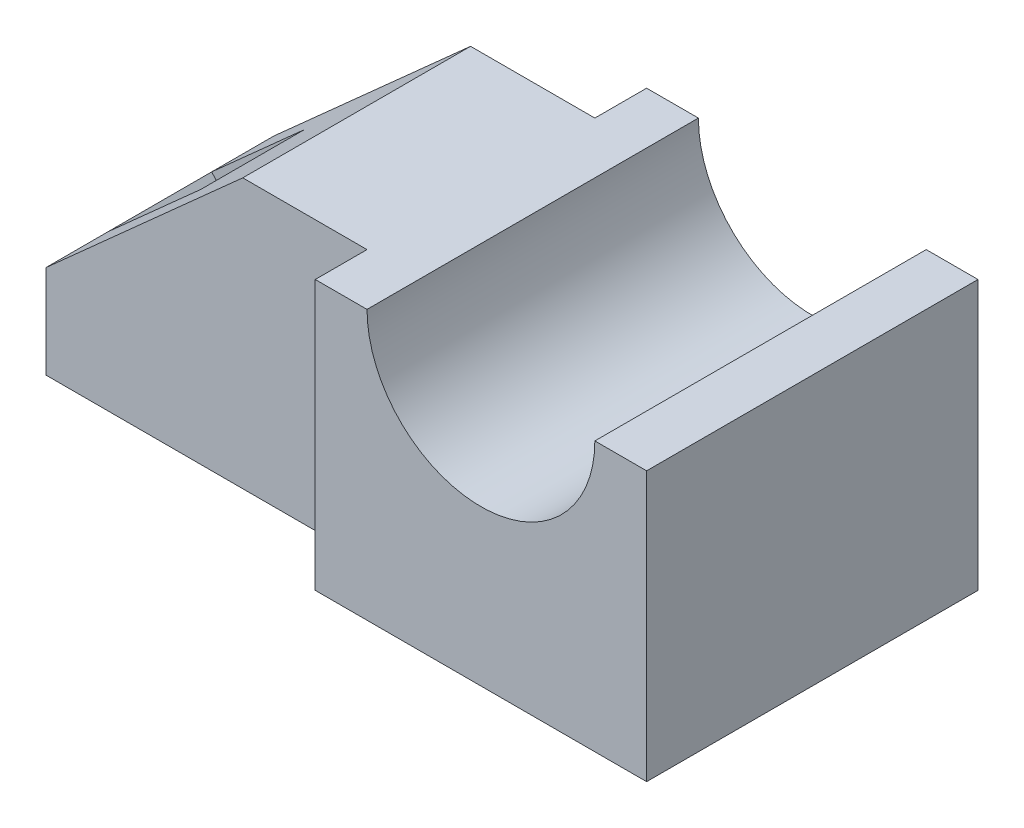
ISO-10303-21;
HEADER;
FILE_DESCRIPTION(('STEP AP214'),'2;1');
FILE_NAME('part.step','',(''),(''),'','','');
FILE_SCHEMA(('AUTOMOTIVE_DESIGN { 1 0 10303 214 1 1 1 1 }'));
ENDSEC;
DATA;
#1=APPLICATION_CONTEXT('core data for automotive mechanical design processes');
#2=APPLICATION_PROTOCOL_DEFINITION('international standard','automotive_design',2000,#1);
#3=PRODUCT_CONTEXT('',#1,'mechanical');
#4=PRODUCT('Part','Part','',(#3));
#5=PRODUCT_RELATED_PRODUCT_CATEGORY('part','',(#4));
#6=PRODUCT_DEFINITION_FORMATION('','',#4);
#7=PRODUCT_DEFINITION_CONTEXT('part definition',#1,'design');
#8=PRODUCT_DEFINITION('design','',#6,#7);
#9=PRODUCT_DEFINITION_SHAPE('','',#8);
#10=(LENGTH_UNIT() NAMED_UNIT(*) SI_UNIT(.MILLI.,.METRE.));
#11=(NAMED_UNIT(*) PLANE_ANGLE_UNIT() SI_UNIT($,.RADIAN.));
#12=(NAMED_UNIT(*) SI_UNIT($,.STERADIAN.) SOLID_ANGLE_UNIT());
#13=UNCERTAINTY_MEASURE_WITH_UNIT(LENGTH_MEASURE(1.E-05),#10,'distance_accuracy_value','');
#14=(GEOMETRIC_REPRESENTATION_CONTEXT(3) GLOBAL_UNCERTAINTY_ASSIGNED_CONTEXT((#13)) GLOBAL_UNIT_ASSIGNED_CONTEXT((#10,
#11,#12)) REPRESENTATION_CONTEXT('',''));
#15=CARTESIAN_POINT('',(0.,0.,0.));
#16=DIRECTION('',(0.,0.,1.));
#17=DIRECTION('',(1.,0.,0.));
#18=AXIS2_PLACEMENT_3D('',#15,#16,#17);
#19=CARTESIAN_POINT('',(-16.,13.,16.));
#20=DIRECTION('',(1.,0.,0.));
#21=DIRECTION('',(0.,1.,0.));
#22=AXIS2_PLACEMENT_3D('',#19,#20,#21);
#23=PLANE('',#22);
#24=DIRECTION('',(0.,1.,0.));
#25=VECTOR('',#24,1.);
#26=CARTESIAN_POINT('',(-16.,13.,11.));
#27=LINE('',#26,#25);
#28=CARTESIAN_POINT('',(-16.,-13.,11.));
#29=VERTEX_POINT('',#28);
#30=CARTESIAN_POINT('',(-16.,13.,11.));
#31=VERTEX_POINT('',#30);
#32=EDGE_CURVE('E285',#29,#31,#27,.T.);
#33=ORIENTED_EDGE('',*,*,#32,.F.);
#34=DIRECTION('',(0.,0.,-1.));
#35=VECTOR('',#34,1.);
#36=CARTESIAN_POINT('',(-16.,-13.,16.));
#37=LINE('',#36,#35);
#38=CARTESIAN_POINT('',(-16.,-13.,16.));
#39=VERTEX_POINT('',#38);
#40=EDGE_CURVE('E220',#39,#29,#37,.T.);
#41=ORIENTED_EDGE('',*,*,#40,.F.);
#42=DIRECTION('',(0.,-1.,0.));
#43=VECTOR('',#42,1.);
#44=CARTESIAN_POINT('',(-16.,13.,16.));
#45=LINE('',#44,#43);
#46=CARTESIAN_POINT('',(-16.,13.,16.));
#47=VERTEX_POINT('',#46);
#48=EDGE_CURVE('E198',#47,#39,#45,.T.);
#49=ORIENTED_EDGE('',*,*,#48,.F.);
#50=DIRECTION('',(0.,0.,-1.));
#51=VECTOR('',#50,1.);
#52=CARTESIAN_POINT('',(-16.,13.,16.));
#53=LINE('',#52,#51);
#54=EDGE_CURVE('E222',#47,#31,#53,.T.);
#55=ORIENTED_EDGE('',*,*,#54,.T.);
#56=EDGE_LOOP('',(#33,#41,#49,#55));
#57=FACE_BOUND('',#56,.T.);
#58=ADVANCED_FACE('F39',(#57),#23,.F.);
#59=CARTESIAN_POINT('',(16.,13.,16.));
#60=DIRECTION('',(-1.,0.,0.));
#61=DIRECTION('',(0.,-1.,0.));
#62=AXIS2_PLACEMENT_3D('',#59,#60,#61);
#63=PLANE('',#62);
#64=DIRECTION('',(0.,1.,0.));
#65=VECTOR('',#64,1.);
#66=CARTESIAN_POINT('',(16.,13.,-16.));
#67=LINE('',#66,#65);
#68=CARTESIAN_POINT('',(16.,-13.,-16.));
#69=VERTEX_POINT('',#68);
#70=CARTESIAN_POINT('',(16.,13.,-16.));
#71=VERTEX_POINT('',#70);
#72=EDGE_CURVE('E179',#69,#71,#67,.T.);
#73=ORIENTED_EDGE('',*,*,#72,.T.);
#74=DIRECTION('',(0.,0.,-1.));
#75=VECTOR('',#74,1.);
#76=CARTESIAN_POINT('',(16.,13.,16.));
#77=LINE('',#76,#75);
#78=CARTESIAN_POINT('',(16.,13.,16.));
#79=VERTEX_POINT('',#78);
#80=EDGE_CURVE('E11',#79,#71,#77,.T.);
#81=ORIENTED_EDGE('',*,*,#80,.F.);
#82=DIRECTION('',(0.,1.,0.));
#83=VECTOR('',#82,1.);
#84=CARTESIAN_POINT('',(16.,13.,16.));
#85=LINE('',#84,#83);
#86=CARTESIAN_POINT('',(16.,-13.,16.));
#87=VERTEX_POINT('',#86);
#88=EDGE_CURVE('E186',#87,#79,#85,.T.);
#89=ORIENTED_EDGE('',*,*,#88,.F.);
#90=DIRECTION('',(0.,0.,-1.));
#91=VECTOR('',#90,1.);
#92=CARTESIAN_POINT('',(16.,-13.,16.));
#93=LINE('',#92,#91);
#94=EDGE_CURVE('E199',#87,#69,#93,.T.);
#95=ORIENTED_EDGE('',*,*,#94,.T.);
#96=EDGE_LOOP('',(#73,#81,#89,#95));
#97=FACE_BOUND('',#96,.T.);
#98=ADVANCED_FACE('F41',(#97),#63,.F.);
#99=CARTESIAN_POINT('',(11.,13.,16.));
#100=DIRECTION('',(0.,-1.,0.));
#101=DIRECTION('',(1.,0.,0.));
#102=AXIS2_PLACEMENT_3D('',#99,#100,#101);
#103=PLANE('',#102);
#104=DIRECTION('',(-1.,0.,0.));
#105=VECTOR('',#104,1.);
#106=CARTESIAN_POINT('',(11.,13.,-16.));
#107=LINE('',#106,#105);
#108=CARTESIAN_POINT('',(11.,13.,-16.));
#109=VERTEX_POINT('',#108);
#110=EDGE_CURVE('E201',#71,#109,#107,.T.);
#111=ORIENTED_EDGE('',*,*,#110,.T.);
#112=DIRECTION('',(0.,0.,-1.));
#113=VECTOR('',#112,1.);
#114=CARTESIAN_POINT('',(11.,13.,16.));
#115=LINE('',#114,#113);
#116=CARTESIAN_POINT('',(11.,13.,16.));
#117=VERTEX_POINT('',#116);
#118=EDGE_CURVE('E50',#117,#109,#115,.T.);
#119=ORIENTED_EDGE('',*,*,#118,.F.);
#120=DIRECTION('',(-1.,0.,0.));
#121=VECTOR('',#120,1.);
#122=CARTESIAN_POINT('',(11.,13.,16.));
#123=LINE('',#122,#121);
#124=EDGE_CURVE('E188',#79,#117,#123,.T.);
#125=ORIENTED_EDGE('',*,*,#124,.F.);
#126=ORIENTED_EDGE('',*,*,#80,.T.);
#127=EDGE_LOOP('',(#111,#119,#125,#126));
#128=FACE_BOUND('',#127,.T.);
#129=ADVANCED_FACE('F252',(#128),#103,.F.);
#130=CARTESIAN_POINT('',(0.,13.,16.));
#131=DIRECTION('',(0.,0.,-1.));
#132=DIRECTION('',(-1.,0.,0.));
#133=AXIS2_PLACEMENT_3D('',#130,#131,#132);
#134=CYLINDRICAL_SURFACE('',#133,11.);
#135=CARTESIAN_POINT('',(0.,13.,-16.));
#136=DIRECTION('',(0.,0.,-1.));
#137=DIRECTION('',(1.,0.,0.));
#138=AXIS2_PLACEMENT_3D('',#135,#136,#137);
#139=CIRCLE('',#138,11.);
#140=CARTESIAN_POINT('',(-11.,13.,-16.));
#141=VERTEX_POINT('',#140);
#142=EDGE_CURVE('E202',#109,#141,#139,.T.);
#143=ORIENTED_EDGE('',*,*,#142,.T.);
#144=DIRECTION('',(0.,0.,-1.));
#145=VECTOR('',#144,1.);
#146=CARTESIAN_POINT('',(-11.,13.,16.));
#147=LINE('',#146,#145);
#148=CARTESIAN_POINT('',(-11.,13.,16.));
#149=VERTEX_POINT('',#148);
#150=EDGE_CURVE('E224',#149,#141,#147,.T.);
#151=ORIENTED_EDGE('',*,*,#150,.F.);
#152=CARTESIAN_POINT('',(0.,13.,16.));
#153=DIRECTION('',(0.,0.,-1.));
#154=DIRECTION('',(1.,0.,0.));
#155=AXIS2_PLACEMENT_3D('',#152,#153,#154);
#156=CIRCLE('',#155,11.);
#157=EDGE_CURVE('E195',#117,#149,#156,.T.);
#158=ORIENTED_EDGE('',*,*,#157,.F.);
#159=ORIENTED_EDGE('',*,*,#118,.T.);
#160=EDGE_LOOP('',(#143,#151,#158,#159));
#161=FACE_BOUND('',#160,.T.);
#162=ADVANCED_FACE('F229',(#161),#134,.F.);
#163=CARTESIAN_POINT('',(-16.,13.,16.));
#164=DIRECTION('',(0.,-1.,0.));
#165=DIRECTION('',(1.,0.,0.));
#166=AXIS2_PLACEMENT_3D('',#163,#164,#165);
#167=PLANE('',#166);
#168=DIRECTION('',(-1.,0.,0.));
#169=VECTOR('',#168,1.);
#170=CARTESIAN_POINT('',(-16.,13.,-16.));
#171=LINE('',#170,#169);
#172=CARTESIAN_POINT('',(-16.,13.,-16.));
#173=VERTEX_POINT('',#172);
#174=EDGE_CURVE('E210',#141,#173,#171,.T.);
#175=ORIENTED_EDGE('',*,*,#174,.T.);
#176=CARTESIAN_POINT('',(-16.,13.,-11.));
#177=VERTEX_POINT('',#176);
#178=EDGE_CURVE('E219',#177,#173,#53,.T.);
#179=ORIENTED_EDGE('',*,*,#178,.F.);
#180=DIRECTION('',(-1.,0.,0.));
#181=VECTOR('',#180,1.);
#182=CARTESIAN_POINT('',(-16.,13.,-11.));
#183=LINE('',#182,#181);
#184=CARTESIAN_POINT('',(-28.,13.,-11.));
#185=VERTEX_POINT('',#184);
#186=EDGE_CURVE('E270',#177,#185,#183,.T.);
#187=ORIENTED_EDGE('',*,*,#186,.T.);
#188=DIRECTION('',(0.,0.,-1.));
#189=VECTOR('',#188,1.);
#190=CARTESIAN_POINT('',(-28.,13.,11.));
#191=LINE('',#190,#189);
#192=CARTESIAN_POINT('',(-28.,13.,11.));
#193=VERTEX_POINT('',#192);
#194=EDGE_CURVE('E178',#193,#185,#191,.T.);
#195=ORIENTED_EDGE('',*,*,#194,.F.);
#196=DIRECTION('',(-1.,0.,0.));
#197=VECTOR('',#196,1.);
#198=CARTESIAN_POINT('',(-16.,13.,11.));
#199=LINE('',#198,#197);
#200=EDGE_CURVE('E283',#31,#193,#199,.T.);
#201=ORIENTED_EDGE('',*,*,#200,.F.);
#202=ORIENTED_EDGE('',*,*,#54,.F.);
#203=DIRECTION('',(-1.,0.,0.));
#204=VECTOR('',#203,1.);
#205=CARTESIAN_POINT('',(-16.,13.,16.));
#206=LINE('',#205,#204);
#207=EDGE_CURVE('E192',#149,#47,#206,.T.);
#208=ORIENTED_EDGE('',*,*,#207,.F.);
#209=ORIENTED_EDGE('',*,*,#150,.T.);
#210=EDGE_LOOP('',(#175,#179,#187,#195,#201,#202,#208,#209));
#211=FACE_BOUND('',#210,.T.);
#212=ADVANCED_FACE('F241',(#211),#167,.F.);
#213=CARTESIAN_POINT('',(-16.,-13.,-11.));
#214=VERTEX_POINT('',#213);
#215=CARTESIAN_POINT('',(-16.,-13.,-16.));
#216=VERTEX_POINT('',#215);
#217=EDGE_CURVE('E216',#214,#216,#37,.T.);
#218=ORIENTED_EDGE('',*,*,#217,.F.);
#219=DIRECTION('',(0.,1.,0.));
#220=VECTOR('',#219,1.);
#221=CARTESIAN_POINT('',(-16.,13.,-11.));
#222=LINE('',#221,#220);
#223=EDGE_CURVE('E264',#214,#177,#222,.T.);
#224=ORIENTED_EDGE('',*,*,#223,.T.);
#225=ORIENTED_EDGE('',*,*,#178,.T.);
#226=DIRECTION('',(0.,-1.,0.));
#227=VECTOR('',#226,1.);
#228=CARTESIAN_POINT('',(-16.,13.,-16.));
#229=LINE('',#228,#227);
#230=EDGE_CURVE('E209',#173,#216,#229,.T.);
#231=ORIENTED_EDGE('',*,*,#230,.T.);
#232=EDGE_LOOP('',(#218,#224,#225,#231));
#233=FACE_BOUND('',#232,.T.);
#234=ADVANCED_FACE('F262',(#233),#23,.F.);
#235=CARTESIAN_POINT('',(-16.,-13.,16.));
#236=DIRECTION('',(0.,1.,0.));
#237=DIRECTION('',(0.,0.,1.));
#238=AXIS2_PLACEMENT_3D('',#235,#236,#237);
#239=PLANE('',#238);
#240=DIRECTION('',(-1.,0.,0.));
#241=VECTOR('',#240,1.);
#242=CARTESIAN_POINT('',(-16.,-13.,-5.));
#243=LINE('',#242,#241);
#244=CARTESIAN_POINT('',(-22.8452015360228,-13.,-5.));
#245=VERTEX_POINT('',#244);
#246=CARTESIAN_POINT('',(-38.9473684210526,-13.,-5.));
#247=VERTEX_POINT('',#246);
#248=EDGE_CURVE('E435',#245,#247,#243,.T.);
#249=ORIENTED_EDGE('',*,*,#248,.T.);
#250=DIRECTION('',(0.,0.,1.));
#251=VECTOR('',#250,1.);
#252=CARTESIAN_POINT('',(-38.9473684210526,-13.,16.));
#253=LINE('',#252,#251);
#254=CARTESIAN_POINT('',(-38.9473684210526,-13.,5.));
#255=VERTEX_POINT('',#254);
#256=EDGE_CURVE('E272',#247,#255,#253,.T.);
#257=ORIENTED_EDGE('',*,*,#256,.T.);
#258=DIRECTION('',(1.,0.,0.));
#259=VECTOR('',#258,1.);
#260=CARTESIAN_POINT('',(-16.,-13.,5.));
#261=LINE('',#260,#259);
#262=CARTESIAN_POINT('',(-22.8452015360228,-13.,5.));
#263=VERTEX_POINT('',#262);
#264=EDGE_CURVE('E155',#255,#263,#261,.T.);
#265=ORIENTED_EDGE('',*,*,#264,.T.);
#266=DIRECTION('',(0.,0.,-1.));
#267=VECTOR('',#266,1.);
#268=CARTESIAN_POINT('',(-22.8452015360228,-13.,16.));
#269=LINE('',#268,#267);
#270=EDGE_CURVE('E268',#263,#245,#269,.T.);
#271=ORIENTED_EDGE('',*,*,#270,.T.);
#272=EDGE_LOOP('',(#249,#257,#265,#271));
#273=FACE_BOUND('',#272,.T.);
#274=DIRECTION('',(1.,0.,0.));
#275=VECTOR('',#274,1.);
#276=CARTESIAN_POINT('',(-16.,-13.,-16.));
#277=LINE('',#276,#275);
#278=EDGE_CURVE('E189',#216,#69,#277,.T.);
#279=ORIENTED_EDGE('',*,*,#278,.T.);
#280=ORIENTED_EDGE('',*,*,#94,.F.);
#281=DIRECTION('',(1.,0.,0.));
#282=VECTOR('',#281,1.);
#283=CARTESIAN_POINT('',(-16.,-13.,16.));
#284=LINE('',#283,#282);
#285=EDGE_CURVE('E196',#39,#87,#284,.T.);
#286=ORIENTED_EDGE('',*,*,#285,.F.);
#287=ORIENTED_EDGE('',*,*,#40,.T.);
#288=DIRECTION('',(1.,0.,0.));
#289=VECTOR('',#288,1.);
#290=CARTESIAN_POINT('',(-47.,-13.,11.));
#291=LINE('',#290,#289);
#292=CARTESIAN_POINT('',(-47.,-13.,11.));
#293=VERTEX_POINT('',#292);
#294=EDGE_CURVE('E277',#293,#29,#291,.T.);
#295=ORIENTED_EDGE('',*,*,#294,.F.);
#296=DIRECTION('',(0.,0.,-1.));
#297=VECTOR('',#296,1.);
#298=CARTESIAN_POINT('',(-47.,-13.,11.));
#299=LINE('',#298,#297);
#300=CARTESIAN_POINT('',(-47.,-13.,-11.));
#301=VERTEX_POINT('',#300);
#302=EDGE_CURVE('E185',#293,#301,#299,.T.);
#303=ORIENTED_EDGE('',*,*,#302,.T.);
#304=DIRECTION('',(1.,0.,0.));
#305=VECTOR('',#304,1.);
#306=CARTESIAN_POINT('',(-47.,-13.,-11.));
#307=LINE('',#306,#305);
#308=EDGE_CURVE('E261',#301,#214,#307,.T.);
#309=ORIENTED_EDGE('',*,*,#308,.T.);
#310=ORIENTED_EDGE('',*,*,#217,.T.);
#311=EDGE_LOOP('',(#279,#280,#286,#287,#295,#303,#309,#310));
#312=FACE_BOUND('',#311,.T.);
#313=ADVANCED_FACE('F258',(#273,#312),#239,.F.);
#314=CARTESIAN_POINT('',(0.,13.,16.));
#315=DIRECTION('',(0.,0.,1.));
#316=DIRECTION('',(1.,0.,0.));
#317=AXIS2_PLACEMENT_3D('',#314,#315,#316);
#318=PLANE('',#317);
#319=ORIENTED_EDGE('',*,*,#88,.T.);
#320=ORIENTED_EDGE('',*,*,#124,.T.);
#321=ORIENTED_EDGE('',*,*,#157,.T.);
#322=ORIENTED_EDGE('',*,*,#207,.T.);
#323=ORIENTED_EDGE('',*,*,#48,.T.);
#324=ORIENTED_EDGE('',*,*,#285,.T.);
#325=EDGE_LOOP('',(#319,#320,#321,#322,#323,#324));
#326=FACE_BOUND('',#325,.T.);
#327=ADVANCED_FACE('F246',(#326),#318,.T.);
#328=CARTESIAN_POINT('',(0.,13.,-16.));
#329=DIRECTION('',(0.,0.,1.));
#330=DIRECTION('',(1.,0.,0.));
#331=AXIS2_PLACEMENT_3D('',#328,#329,#330);
#332=PLANE('',#331);
#333=ORIENTED_EDGE('',*,*,#72,.F.);
#334=ORIENTED_EDGE('',*,*,#278,.F.);
#335=ORIENTED_EDGE('',*,*,#230,.F.);
#336=ORIENTED_EDGE('',*,*,#174,.F.);
#337=ORIENTED_EDGE('',*,*,#142,.F.);
#338=ORIENTED_EDGE('',*,*,#110,.F.);
#339=EDGE_LOOP('',(#333,#334,#335,#336,#337,#338));
#340=FACE_BOUND('',#339,.T.);
#341=ADVANCED_FACE('F237',(#340),#332,.F.);
#342=CARTESIAN_POINT('',(-28.,13.,11.));
#343=DIRECTION('',(0.666794859469826,-0.745241313525099,0.));
#344=DIRECTION('',(0.745241313525099,0.666794859469826,0.));
#345=AXIS2_PLACEMENT_3D('',#342,#343,#344);
#346=PLANE('',#345);
#347=DIRECTION('',(0.,0.,-1.));
#348=VECTOR('',#347,1.);
#349=CARTESIAN_POINT('',(-47.,-4.,11.));
#350=LINE('',#349,#348);
#351=CARTESIAN_POINT('',(-47.,-4.,-5.));
#352=VERTEX_POINT('',#351);
#353=CARTESIAN_POINT('',(-47.,-4.,-11.));
#354=VERTEX_POINT('',#353);
#355=EDGE_CURVE('E180',#352,#354,#350,.T.);
#356=ORIENTED_EDGE('',*,*,#355,.F.);
#357=DIRECTION('',(-0.745241313525099,-0.666794859469826,0.));
#358=VECTOR('',#357,1.);
#359=CARTESIAN_POINT('',(-47.,-4.00000000000001,-5.));
#360=LINE('',#359,#358);
#361=CARTESIAN_POINT('',(-38.0571042376988,4.00153831363791,-5.));
#362=VERTEX_POINT('',#361);
#363=EDGE_CURVE('E65',#362,#352,#360,.T.);
#364=ORIENTED_EDGE('',*,*,#363,.F.);
#365=DIRECTION('',(0.,0.,-1.));
#366=VECTOR('',#365,1.);
#367=CARTESIAN_POINT('',(-38.0571042376988,4.00153831363791,-5.));
#368=LINE('',#367,#366);
#369=CARTESIAN_POINT('',(-38.0571042376988,4.00153831363791,5.));
#370=VERTEX_POINT('',#369);
#371=EDGE_CURVE('E171',#370,#362,#368,.T.);
#372=ORIENTED_EDGE('',*,*,#371,.F.);
#373=DIRECTION('',(0.745241313525099,0.666794859469826,0.));
#374=VECTOR('',#373,1.);
#375=CARTESIAN_POINT('',(-38.0571042376988,4.00153831363791,5.));
#376=LINE('',#375,#374);
#377=CARTESIAN_POINT('',(-47.,-4.00000000000001,5.));
#378=VERTEX_POINT('',#377);
#379=EDGE_CURVE('E149',#378,#370,#376,.T.);
#380=ORIENTED_EDGE('',*,*,#379,.F.);
#381=CARTESIAN_POINT('',(-47.,-4.,11.));
#382=VERTEX_POINT('',#381);
#383=EDGE_CURVE('E169',#382,#378,#350,.T.);
#384=ORIENTED_EDGE('',*,*,#383,.F.);
#385=DIRECTION('',(-0.745241313525099,-0.666794859469826,0.));
#386=VECTOR('',#385,1.);
#387=CARTESIAN_POINT('',(-28.,13.,11.));
#388=LINE('',#387,#386);
#389=EDGE_CURVE('E286',#193,#382,#388,.T.);
#390=ORIENTED_EDGE('',*,*,#389,.F.);
#391=ORIENTED_EDGE('',*,*,#194,.T.);
#392=DIRECTION('',(-0.745241313525099,-0.666794859469826,0.));
#393=VECTOR('',#392,1.);
#394=CARTESIAN_POINT('',(-28.,13.,-11.));
#395=LINE('',#394,#393);
#396=EDGE_CURVE('E269',#185,#354,#395,.T.);
#397=ORIENTED_EDGE('',*,*,#396,.T.);
#398=EDGE_LOOP('',(#356,#364,#372,#380,#384,#390,#391,#397));
#399=FACE_BOUND('',#398,.T.);
#400=ADVANCED_FACE('F167',(#399),#346,.F.);
#401=CARTESIAN_POINT('',(-47.,-4.,11.));
#402=DIRECTION('',(1.,0.,0.));
#403=DIRECTION('',(0.,0.,-1.));
#404=AXIS2_PLACEMENT_3D('',#401,#402,#403);
#405=PLANE('',#404);
#406=DIRECTION('',(0.,-1.,0.));
#407=VECTOR('',#406,1.);
#408=CARTESIAN_POINT('',(-47.,-4.,-11.));
#409=LINE('',#408,#407);
#410=EDGE_CURVE('E281',#354,#301,#409,.T.);
#411=ORIENTED_EDGE('',*,*,#410,.T.);
#412=ORIENTED_EDGE('',*,*,#302,.F.);
#413=DIRECTION('',(0.,-1.,0.));
#414=VECTOR('',#413,1.);
#415=CARTESIAN_POINT('',(-47.,-4.,11.));
#416=LINE('',#415,#414);
#417=EDGE_CURVE('E174',#382,#293,#416,.T.);
#418=ORIENTED_EDGE('',*,*,#417,.F.);
#419=ORIENTED_EDGE('',*,*,#383,.T.);
#420=DIRECTION('',(0.,0.,1.));
#421=VECTOR('',#420,1.);
#422=CARTESIAN_POINT('',(-47.,-4.00000000000001,-5.));
#423=LINE('',#422,#421);
#424=EDGE_CURVE('E160',#352,#378,#423,.T.);
#425=ORIENTED_EDGE('',*,*,#424,.F.);
#426=ORIENTED_EDGE('',*,*,#355,.T.);
#427=EDGE_LOOP('',(#411,#412,#418,#419,#425,#426));
#428=FACE_BOUND('',#427,.T.);
#429=ADVANCED_FACE('F172',(#428),#405,.F.);
#430=CARTESIAN_POINT('',(0.,0.,11.));
#431=DIRECTION('',(0.,0.,1.));
#432=DIRECTION('',(1.,0.,0.));
#433=AXIS2_PLACEMENT_3D('',#430,#431,#432);
#434=PLANE('',#433);
#435=ORIENTED_EDGE('',*,*,#32,.T.);
#436=ORIENTED_EDGE('',*,*,#200,.T.);
#437=ORIENTED_EDGE('',*,*,#389,.T.);
#438=ORIENTED_EDGE('',*,*,#417,.T.);
#439=ORIENTED_EDGE('',*,*,#294,.T.);
#440=EDGE_LOOP('',(#435,#436,#437,#438,#439));
#441=FACE_BOUND('',#440,.T.);
#442=ADVANCED_FACE('F300',(#441),#434,.T.);
#443=CARTESIAN_POINT('',(0.,0.,-11.));
#444=DIRECTION('',(0.,0.,1.));
#445=DIRECTION('',(1.,0.,0.));
#446=AXIS2_PLACEMENT_3D('',#443,#444,#445);
#447=PLANE('',#446);
#448=ORIENTED_EDGE('',*,*,#223,.F.);
#449=ORIENTED_EDGE('',*,*,#308,.F.);
#450=ORIENTED_EDGE('',*,*,#410,.F.);
#451=ORIENTED_EDGE('',*,*,#396,.F.);
#452=ORIENTED_EDGE('',*,*,#186,.F.);
#453=EDGE_LOOP('',(#448,#449,#450,#451,#452));
#454=FACE_BOUND('',#453,.T.);
#455=ADVANCED_FACE('F294',(#454),#447,.F.);
#456=CARTESIAN_POINT('',(-5.57402731462186,-32.3030770709775,-5.));
#457=DIRECTION('',(0.745241313525099,0.666794859469826,0.));
#458=DIRECTION('',(-0.666794859469826,0.745241313525099,0.));
#459=AXIS2_PLACEMENT_3D('',#456,#457,#458);
#460=PLANE('',#459);
#461=DIRECTION('',(-0.666794859469826,0.745241313525099,0.));
#462=VECTOR('',#461,1.);
#463=CARTESIAN_POINT('',(-5.57402731462186,-32.3030770709775,5.));
#464=LINE('',#463,#462);
#465=EDGE_CURVE('E53',#263,#370,#464,.T.);
#466=ORIENTED_EDGE('',*,*,#465,.T.);
#467=ORIENTED_EDGE('',*,*,#371,.T.);
#468=DIRECTION('',(-0.666794859469826,0.745241313525099,0.));
#469=VECTOR('',#468,1.);
#470=CARTESIAN_POINT('',(-5.57402731462186,-32.3030770709775,-5.));
#471=LINE('',#470,#469);
#472=EDGE_CURVE('E429',#245,#362,#471,.T.);
#473=ORIENTED_EDGE('',*,*,#472,.F.);
#474=ORIENTED_EDGE('',*,*,#270,.F.);
#475=EDGE_LOOP('',(#466,#467,#473,#474));
#476=FACE_BOUND('',#475,.T.);
#477=ADVANCED_FACE('F302',(#476),#460,.F.);
#478=CARTESIAN_POINT('',(-14.516923076923,-40.3046153846154,-5.));
#479=DIRECTION('',(-0.745241313525099,-0.666794859469826,0.));
#480=DIRECTION('',(0.666794859469826,-0.745241313525099,0.));
#481=AXIS2_PLACEMENT_3D('',#478,#479,#480);
#482=PLANE('',#481);
#483=DIRECTION('',(-0.666794859469826,0.745241313525099,0.));
#484=VECTOR('',#483,1.);
#485=CARTESIAN_POINT('',(-14.516923076923,-40.3046153846154,-5.));
#486=LINE('',#485,#484);
#487=EDGE_CURVE('E157',#247,#352,#486,.T.);
#488=ORIENTED_EDGE('',*,*,#487,.T.);
#489=ORIENTED_EDGE('',*,*,#424,.T.);
#490=DIRECTION('',(-0.666794859469826,0.745241313525099,0.));
#491=VECTOR('',#490,1.);
#492=CARTESIAN_POINT('',(-14.516923076923,-40.3046153846154,5.));
#493=LINE('',#492,#491);
#494=EDGE_CURVE('E144',#255,#378,#493,.T.);
#495=ORIENTED_EDGE('',*,*,#494,.F.);
#496=ORIENTED_EDGE('',*,*,#256,.F.);
#497=EDGE_LOOP('',(#488,#489,#495,#496));
#498=FACE_BOUND('',#497,.T.);
#499=ADVANCED_FACE('F158',(#498),#482,.F.);
#500=CARTESIAN_POINT('',(-14.516923076923,-40.3046153846154,-5.));
#501=DIRECTION('',(0.,0.,-1.));
#502=DIRECTION('',(-1.,0.,0.));
#503=AXIS2_PLACEMENT_3D('',#500,#501,#502);
#504=PLANE('',#503);
#505=ORIENTED_EDGE('',*,*,#472,.T.);
#506=ORIENTED_EDGE('',*,*,#363,.T.);
#507=ORIENTED_EDGE('',*,*,#487,.F.);
#508=ORIENTED_EDGE('',*,*,#248,.F.);
#509=EDGE_LOOP('',(#505,#506,#507,#508));
#510=FACE_BOUND('',#509,.T.);
#511=ADVANCED_FACE('F413',(#510),#504,.F.);
#512=CARTESIAN_POINT('',(-5.57402731462186,-32.3030770709775,5.));
#513=DIRECTION('',(0.,0.,1.));
#514=DIRECTION('',(1.,0.,0.));
#515=AXIS2_PLACEMENT_3D('',#512,#513,#514);
#516=PLANE('',#515);
#517=ORIENTED_EDGE('',*,*,#494,.T.);
#518=ORIENTED_EDGE('',*,*,#379,.T.);
#519=ORIENTED_EDGE('',*,*,#465,.F.);
#520=ORIENTED_EDGE('',*,*,#264,.F.);
#521=EDGE_LOOP('',(#517,#518,#519,#520));
#522=FACE_BOUND('',#521,.T.);
#523=ADVANCED_FACE('F150',(#522),#516,.F.);
#524=CLOSED_SHELL('',(#58,#98,#129,#162,#212,#234,#313,#327,#341,#400,#429,#442,#455,#477,#499,
#511,#523));
#525=MANIFOLD_SOLID_BREP('B2',#524);
#526=ADVANCED_BREP_SHAPE_REPRESENTATION('',(#18,#525),#14);
#527=SHAPE_DEFINITION_REPRESENTATION(#9,#526);
ENDSEC;
END-ISO-10303-21;
